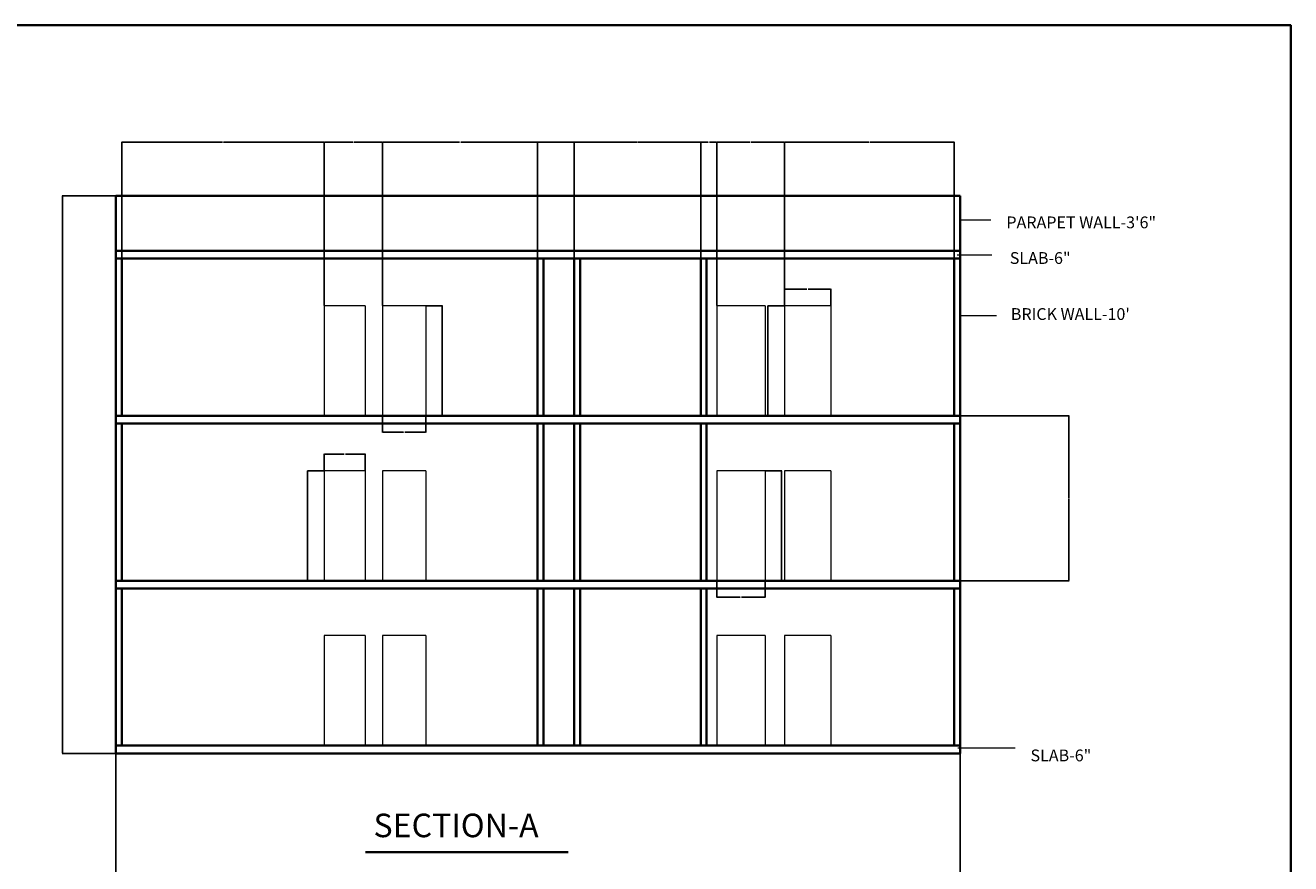
# Model space of a CAD drawing. Units: inches. Extents: x 1520 to 3401, y 1570 to 3432.
# Tile 15 of 15: x 2435 to 3401, y 2791 to 3432. Entities that reach past the tile are written whole.
import ezdxf

# ---------------------------------------------------------------- set-up
doc = ezdxf.new("R2010")
doc.units = ezdxf.units.IN
for name, color, linetype, lineweight in [('A-ANNO-DIMS', 2, 'Continuous', 18), ('A-ANNO-TEXT', 7, 'Continuous', 18), ('A-ANNO-TITL', 7, 'Continuous', 35), ('A-ANNO-TTLB', 7, 'Continuous', 35), ('A-SECT', 7, 'Continuous', 35), ('A-SECT-DOOR', 3, 'Continuous', 18), ('A-SECT-SLAB', 7, 'Continuous', 35)]:
    doc.layers.add(name, color=color, linetype=linetype, lineweight=lineweight)
doc.styles.get("Standard").update_dxf_attribs({"font": 'arial.ttf'})
doc.dimstyles.get("Standard").update_dxf_attribs({"dimtxt": 0.18, "dimasz": 0.18, "dimexe": 0.18, "dimexo": 0.0625, "dimgap": 0.09, "dimtad": 0, "dimtih": 1, "dimtoh": 1, "dimdec": 4, "dimzin": 0, "dimdsep": 46, "dimtxsty": 'Standard', "dimcen": 0.09, "dimadec": 0, "dimazin": 0, "dimtfac": 1, "dimtdec": 4, "dimtofl": 0, "dimtmove": 0, "dimatfit": 3, "dimfxl": 1, "dimtolj": 1, "dimtzin": 0, "dimarcsym": 0})

# ---------------------------------------------------------------- blocks, each defined once
blk = doc.blocks.new('DOOR-SECT-01')
for p, q in [((0, 84), (0, 0)), ((31.45, 84), (0, 84)), ((31.45, 84), (31.45, 0))]:
    blk.add_line(p, q)
blk = doc.blocks.new('DOOR-SECT-02')
for p, q in [((0, 84), (0, 0)), ((32.99, 84), (0, 84)), ((32.99, 84), (32.99, 0))]:
    blk.add_line(p, q)
blk = doc.blocks.new('DOOR-SECT-03')
for p, q in [((0, 84), (0, 0)), ((36.83, 84), (0, 84)), ((36.83, 84), (36.83, 0))]:
    blk.add_line(p, q)
blk = doc.blocks.new('DOOR-SECT-04')
for p, q in [((0, 84), (0, 0)), ((35.31, 84), (0, 84)), ((35.31, 84), (35.31, 0))]:
    blk.add_line(p, q)
blk = doc.blocks.new('*D73')
at = {"layer": 'A-ANNO-DIMS', "color": 0, "lineweight": -2, "transparency": 16777216}
for p, q in [((2662.81, 3091.63), (2650.09, 3091.63)), ((2650.27, 3091.45), (2650.27, 3049.82)), ((2650.27, 3007.81), (2650.27, 3049.45)), ((2662.81, 3007.63), (2650.09, 3007.63))]:
    blk.add_line(p, q, dxfattribs=at)
at = {"layer": 'A-ANNO-DIMS', "color": 0, "transparency": 16777216}
for points in [[(2650.24, 3091.45), (2650.3, 3091.45), (2650.27, 3091.63)], [(2650.24, 3007.81), (2650.3, 3007.81), (2650.27, 3007.63)]]:
    blk.add_solid(points, dxfattribs=at)
at = {"layer": 'Defpoints', "color": 0, "transparency": 16777216}
for p in [(2650.27, 3091.63), (2662.87, 3091.63), (2662.87, 3007.63)]:
    blk.add_point(p, dxfattribs=at)
at = {"layer": 'A-ANNO-DIMS', "color": 0, "transparency": 16777216, "insert": (2650.27, 3049.63), "char_height": 0.18, "attachment_point": 5}
blk.add_mtext('\\A1;S1 84 TYP.', dxfattribs=at)
blk = doc.blocks.new('*D74')
at = {"layer": 'A-ANNO-DIMS', "color": 0, "lineweight": -2, "transparency": 16777216}
for p, q in [((2662.87, 3091.7), (2662.87, 3104.41)), ((2663.05, 3104.23), (2678.07, 3104.23)), ((2694.14, 3104.23), (2679.12, 3104.23)), ((2694.32, 3091.7), (2694.32, 3104.41))]:
    blk.add_line(p, q, dxfattribs=at)
at = {"layer": 'A-ANNO-DIMS', "color": 0, "transparency": 16777216}
for points in [[(2663.05, 3104.26), (2663.05, 3104.2), (2662.87, 3104.23)], [(2694.14, 3104.26), (2694.14, 3104.2), (2694.32, 3104.23)]]:
    blk.add_solid(points, dxfattribs=at)
at = {"layer": 'Defpoints', "color": 0, "transparency": 16777216}
for p in [(2694.32, 3104.23), (2662.87, 3091.63), (2694.32, 3091.63)]:
    blk.add_point(p, dxfattribs=at)
at = {"layer": 'A-ANNO-DIMS', "color": 0, "transparency": 16777216, "insert": (2678.6, 3104.23), "char_height": 0.18, "attachment_point": 5}
blk.add_mtext('\\A1;31 TYP.', dxfattribs=at)
blk = doc.blocks.new('*D75')
at = {"layer": 'A-ANNO-DIMS', "color": 0, "lineweight": -2, "transparency": 16777216}
for p, q in [((2740.5, 3217.63), (2753.22, 3217.63)), ((2753.04, 3217.45), (2753.04, 3175.82)), ((2753.04, 3133.81), (2753.04, 3175.45)), ((2740.5, 3133.63), (2753.22, 3133.63))]:
    blk.add_line(p, q, dxfattribs=at)
at = {"layer": 'A-ANNO-DIMS', "color": 0, "transparency": 16777216}
for points in [[(2753.01, 3217.45), (2753.07, 3217.45), (2753.04, 3217.63)], [(2753.01, 3133.81), (2753.07, 3133.81), (2753.04, 3133.63)]]:
    blk.add_solid(points, dxfattribs=at)
at = {"layer": 'Defpoints', "color": 0, "transparency": 16777216}
for p in [(2740.44, 3217.63), (2753.04, 3217.63), (2740.44, 3133.63)]:
    blk.add_point(p, dxfattribs=at)
at = {"layer": 'A-ANNO-DIMS', "color": 0, "transparency": 16777216, "insert": (2753.04, 3175.63), "char_height": 0.18, "attachment_point": 5}
blk.add_mtext('\\A1;S2 84 TYP.', dxfattribs=at)
blk = doc.blocks.new('*D76')
at = {"layer": 'A-ANNO-DIMS', "color": 0, "lineweight": -2, "transparency": 16777216}
for p, q in [((2707.45, 3133.57), (2707.45, 3120.85)), ((2740.44, 3133.57), (2740.44, 3120.85)), ((2707.63, 3121.03), (2723.42, 3121.03)), ((2740.26, 3121.03), (2724.47, 3121.03))]:
    blk.add_line(p, q, dxfattribs=at)
at = {"layer": 'A-ANNO-DIMS', "color": 0, "transparency": 16777216}
for points in [[(2707.63, 3121.06), (2707.63, 3121), (2707.45, 3121.03)], [(2740.26, 3121.06), (2740.26, 3121), (2740.44, 3121.03)]]:
    blk.add_solid(points, dxfattribs=at)
at = {"layer": 'Defpoints', "color": 0, "transparency": 16777216}
for p in [(2707.45, 3133.63), (2740.44, 3133.63), (2740.44, 3121.03)]:
    blk.add_point(p, dxfattribs=at)
at = {"layer": 'A-ANNO-DIMS', "color": 0, "transparency": 16777216, "insert": (2723.95, 3121.03), "char_height": 0.18, "attachment_point": 5}
blk.add_mtext('\\A1;33 TYP.', dxfattribs=at)
blk = doc.blocks.new('*D77')
at = {"layer": 'A-ANNO-DIMS', "color": 0, "lineweight": -2, "transparency": 16777216}
for p, q in [((2999.61, 3091.63), (3012.33, 3091.63)), ((3012.15, 3091.45), (3012.15, 3049.82)), ((3012.15, 3007.81), (3012.15, 3049.45)), ((2999.61, 3007.63), (3012.33, 3007.63))]:
    blk.add_line(p, q, dxfattribs=at)
at = {"layer": 'A-ANNO-DIMS', "color": 0, "transparency": 16777216}
for points in [[(3012.12, 3091.45), (3012.18, 3091.45), (3012.15, 3091.63)], [(3012.12, 3007.81), (3012.18, 3007.81), (3012.15, 3007.63)]]:
    blk.add_solid(points, dxfattribs=at)
at = {"layer": 'Defpoints', "color": 0, "transparency": 16777216}
for p in [(2999.55, 3091.63), (3012.15, 3091.63), (2999.55, 3007.63)]:
    blk.add_point(p, dxfattribs=at)
at = {"layer": 'A-ANNO-DIMS', "color": 0, "transparency": 16777216, "insert": (3012.15, 3049.63), "char_height": 0.18, "attachment_point": 5}
blk.add_mtext('\\A1;S3 84 TYP.', dxfattribs=at)
blk = doc.blocks.new('*D78')
at = {"layer": 'A-ANNO-DIMS', "color": 0, "lineweight": -2, "transparency": 16777216}
for p, q in [((2962.72, 3007.57), (2962.72, 2994.85)), ((2999.55, 3007.57), (2999.55, 2994.85)), ((2962.9, 2995.03), (2980.61, 2995.03)), ((2999.37, 2995.03), (2981.66, 2995.03))]:
    blk.add_line(p, q, dxfattribs=at)
at = {"layer": 'A-ANNO-DIMS', "color": 0, "transparency": 16777216}
for points in [[(2962.9, 2995.06), (2962.9, 2995), (2962.72, 2995.03)], [(2999.37, 2995.06), (2999.37, 2995), (2999.55, 2995.03)]]:
    blk.add_solid(points, dxfattribs=at)
at = {"layer": 'Defpoints', "color": 0, "transparency": 16777216}
for p in [(2962.72, 3007.63), (2999.55, 3007.63), (2999.55, 2995.03)]:
    blk.add_point(p, dxfattribs=at)
at = {"layer": 'A-ANNO-DIMS', "color": 0, "transparency": 16777216, "insert": (2981.14, 2995.03), "char_height": 0.18, "attachment_point": 5}
blk.add_mtext('\\A1;37 TYP.', dxfattribs=at)
blk = doc.blocks.new('*D79')
at = {"layer": 'A-ANNO-DIMS', "color": 0, "lineweight": -2, "transparency": 16777216}
for p, q in [((3014.28, 3217.63), (3001.56, 3217.63)), ((3001.74, 3217.45), (3001.74, 3175.82)), ((3001.74, 3133.81), (3001.74, 3175.45)), ((3014.28, 3133.63), (3001.56, 3133.63))]:
    blk.add_line(p, q, dxfattribs=at)
at = {"layer": 'A-ANNO-DIMS', "color": 0, "transparency": 16777216}
for points in [[(3001.71, 3217.45), (3001.77, 3217.45), (3001.74, 3217.63)], [(3001.71, 3133.81), (3001.77, 3133.81), (3001.74, 3133.63)]]:
    blk.add_solid(points, dxfattribs=at)
at = {"layer": 'Defpoints', "color": 0, "transparency": 16777216}
for p in [(3001.74, 3217.63), (3014.34, 3217.63), (3014.34, 3133.63)]:
    blk.add_point(p, dxfattribs=at)
at = {"layer": 'A-ANNO-DIMS', "color": 0, "transparency": 16777216, "insert": (3001.74, 3175.63), "char_height": 0.18, "attachment_point": 5}
blk.add_mtext('\\A1;S4 84 TYP.', dxfattribs=at)
blk = doc.blocks.new('*D80')
at = {"layer": 'A-ANNO-DIMS', "color": 0, "lineweight": -2, "transparency": 16777216}
for p, q in [((3014.34, 3217.7), (3014.34, 3230.41)), ((3014.52, 3230.23), (3031.47, 3230.23)), ((3049.47, 3230.23), (3032.52, 3230.23)), ((3049.65, 3217.7), (3049.65, 3230.41))]:
    blk.add_line(p, q, dxfattribs=at)
at = {"layer": 'A-ANNO-DIMS', "color": 0, "transparency": 16777216}
for points in [[(3014.52, 3230.26), (3014.52, 3230.2), (3014.34, 3230.23)], [(3049.47, 3230.26), (3049.47, 3230.2), (3049.65, 3230.23)]]:
    blk.add_solid(points, dxfattribs=at)
at = {"layer": 'Defpoints', "color": 0, "transparency": 16777216}
for p in [(3049.65, 3230.23), (3014.34, 3217.63), (3049.65, 3217.63)]:
    blk.add_point(p, dxfattribs=at)
at = {"layer": 'A-ANNO-DIMS', "color": 0, "transparency": 16777216, "insert": (3032, 3230.23), "char_height": 0.18, "attachment_point": 5}
blk.add_mtext('\\A1;35 TYP.', dxfattribs=at)
blk = doc.blocks.new('*D211')
at = {"layer": 'A-ANNO-DIMS', "color": 0, "lineweight": -2, "transparency": 16777216}
for p, q in [((3148.46, 3133.63), (3231.65, 3133.63)), ((3231.47, 3133.45), (3231.47, 3070.81)), ((3231.47, 3007.81), (3231.47, 3070.45)), ((3148.46, 3007.63), (3231.65, 3007.63))]:
    blk.add_line(p, q, dxfattribs=at)
at = {"layer": 'A-ANNO-DIMS', "color": 0, "transparency": 16777216}
for points in [[(3231.44, 3133.45), (3231.5, 3133.45), (3231.47, 3133.63)], [(3231.44, 3007.81), (3231.5, 3007.81), (3231.47, 3007.63)]]:
    blk.add_solid(points, dxfattribs=at)
at = {"layer": 'Defpoints', "color": 0, "transparency": 16777216}
for p in [(3148.4, 3133.63), (3231.47, 3133.63), (3148.4, 3007.63)]:
    blk.add_point(p, dxfattribs=at)
at = {"layer": 'A-ANNO-DIMS', "color": 0, "transparency": 16777216, "insert": (3231.47, 3070.63), "char_height": 0.18, "attachment_point": 5}
blk.add_mtext('\\A1;126', dxfattribs=at)
blk = doc.blocks.new('*D224')
at = {"layer": 'A-ANNO-DIMS', "color": 0, "lineweight": -2, "transparency": 16777216}
for p, q in [((2503.9, 2875.57), (2503.9, 2759.2)), ((3148.4, 2875.57), (3148.4, 2759.2)), ((2504.08, 2759.38), (2825.75, 2759.38)), ((3148.22, 2759.38), (2826.54, 2759.38))]:
    blk.add_line(p, q, dxfattribs=at)
at = {"layer": 'A-ANNO-DIMS', "color": 0, "transparency": 16777216}
for points in [[(2504.08, 2759.41), (2504.08, 2759.35), (2503.9, 2759.38)], [(3148.22, 2759.41), (3148.22, 2759.35), (3148.4, 2759.38)]]:
    blk.add_solid(points, dxfattribs=at)
at = {"layer": 'Defpoints', "color": 0, "transparency": 16777216}
for p in [(2503.9, 2875.63), (3148.4, 2875.63), (3148.4, 2759.38)]:
    blk.add_point(p, dxfattribs=at)
at = {"layer": 'A-ANNO-DIMS', "color": 0, "transparency": 16777216, "insert": (2826.15, 2759.38), "char_height": 0.18, "attachment_point": 5}
blk.add_mtext('\\A1;644.5', dxfattribs=at)
blk = doc.blocks.new('*D225')
at = {"layer": 'A-ANNO-DIMS', "color": 0, "lineweight": -2, "transparency": 16777216}
for p, q in [((2503.84, 3301.63), (2462.87, 3301.63)), ((2463.05, 3301.45), (2463.05, 3088.81)), ((2463.05, 2875.81), (2463.05, 3088.45)), ((2503.84, 2875.63), (2462.87, 2875.63))]:
    blk.add_line(p, q, dxfattribs=at)
at = {"layer": 'A-ANNO-DIMS', "color": 0, "transparency": 16777216}
for points in [[(2463.02, 3301.45), (2463.08, 3301.45), (2463.05, 3301.63)], [(2463.02, 2875.81), (2463.08, 2875.81), (2463.05, 2875.63)]]:
    blk.add_solid(points, dxfattribs=at)
at = {"layer": 'Defpoints', "color": 0, "transparency": 16777216}
for p in [(2503.9, 3301.63), (2463.05, 2875.63), (2503.9, 2875.63)]:
    blk.add_point(p, dxfattribs=at)
at = {"layer": 'A-ANNO-DIMS', "color": 0, "transparency": 16777216, "insert": (2463.05, 3088.63), "char_height": 0.18, "attachment_point": 5}
blk.add_mtext('\\A1;426', dxfattribs=at)
blk = doc.blocks.new('*D226')
at = {"layer": 'A-ANNO-DIMS', "color": 0, "lineweight": -2, "transparency": 16777216}
for p, q in [((2508.4, 3253.7), (2508.4, 3342.66)), ((2508.58, 3342.48), (2585.18, 3342.48)), ((2662.69, 3342.48), (2586.09, 3342.48)), ((2662.87, 3217.7), (2662.87, 3342.66))]:
    blk.add_line(p, q, dxfattribs=at)
at = {"layer": 'A-ANNO-DIMS', "color": 0, "transparency": 16777216}
for points in [[(2508.58, 3342.51), (2508.58, 3342.45), (2508.4, 3342.48)], [(2662.69, 3342.51), (2662.69, 3342.45), (2662.87, 3342.48)]]:
    blk.add_solid(points, dxfattribs=at)
at = {"layer": 'Defpoints', "color": 0, "transparency": 16777216}
for p in [(2662.87, 3342.48), (2508.4, 3253.63), (2662.87, 3217.63)]:
    blk.add_point(p, dxfattribs=at)
at = {"layer": 'A-ANNO-DIMS', "color": 0, "transparency": 16777216, "insert": (2585.64, 3342.48), "char_height": 0.18, "attachment_point": 5}
blk.add_mtext('\\A1;154.47', dxfattribs=at)
blk = doc.blocks.new('*D227')
at = {"layer": 'A-ANNO-DIMS', "color": 0, "lineweight": -2, "transparency": 16777216}
for p, q in [((2662.87, 3217.7), (2662.87, 3342.66)), ((2663.05, 3342.48), (2684.76, 3342.48)), ((2707.27, 3342.48), (2685.56, 3342.48)), ((2707.45, 3217.7), (2707.45, 3342.66))]:
    blk.add_line(p, q, dxfattribs=at)
at = {"layer": 'A-ANNO-DIMS', "color": 0, "transparency": 16777216}
for points in [[(2663.05, 3342.51), (2663.05, 3342.45), (2662.87, 3342.48)], [(2707.27, 3342.51), (2707.27, 3342.45), (2707.45, 3342.48)]]:
    blk.add_solid(points, dxfattribs=at)
at = {"layer": 'Defpoints', "color": 0, "transparency": 16777216}
for p in [(2707.45, 3342.48), (2662.87, 3217.63), (2707.45, 3217.63)]:
    blk.add_point(p, dxfattribs=at)
at = {"layer": 'A-ANNO-DIMS', "color": 0, "transparency": 16777216, "insert": (2685.16, 3342.48), "char_height": 0.18, "attachment_point": 5}
blk.add_mtext('\\A1;44.58', dxfattribs=at)
blk = doc.blocks.new('*D228')
at = {"layer": 'A-ANNO-DIMS', "color": 0, "lineweight": -2, "transparency": 16777216}
for p, q in [((2707.45, 3217.7), (2707.45, 3342.66)), ((2707.63, 3342.48), (2766.22, 3342.48)), ((2825.72, 3342.48), (2767.13, 3342.48)), ((2825.9, 3253.7), (2825.9, 3342.66))]:
    blk.add_line(p, q, dxfattribs=at)
at = {"layer": 'A-ANNO-DIMS', "color": 0, "transparency": 16777216}
for points in [[(2707.63, 3342.51), (2707.63, 3342.45), (2707.45, 3342.48)], [(2825.72, 3342.51), (2825.72, 3342.45), (2825.9, 3342.48)]]:
    blk.add_solid(points, dxfattribs=at)
at = {"layer": 'Defpoints', "color": 0, "transparency": 16777216}
for p in [(2825.9, 3342.48), (2825.9, 3253.63), (2707.45, 3217.63)]:
    blk.add_point(p, dxfattribs=at)
at = {"layer": 'A-ANNO-DIMS', "color": 0, "transparency": 16777216, "insert": (2766.67, 3342.48), "char_height": 0.18, "attachment_point": 5}
blk.add_mtext('\\A1;118.45', dxfattribs=at)
blk = doc.blocks.new('*D229')
at = {"layer": 'A-ANNO-DIMS', "color": 0, "lineweight": -2, "transparency": 16777216}
for p, q in [((2825.9, 3253.7), (2825.9, 3342.66)), ((2826.08, 3342.48), (2839.68, 3342.48)), ((2853.72, 3342.48), (2840.12, 3342.48)), ((2853.9, 3253.7), (2853.9, 3342.66))]:
    blk.add_line(p, q, dxfattribs=at)
at = {"layer": 'A-ANNO-DIMS', "color": 0, "transparency": 16777216}
for points in [[(2826.08, 3342.51), (2826.08, 3342.45), (2825.9, 3342.48)], [(2853.72, 3342.51), (2853.72, 3342.45), (2853.9, 3342.48)]]:
    blk.add_solid(points, dxfattribs=at)
at = {"layer": 'Defpoints', "color": 0, "transparency": 16777216}
for p in [(2853.9, 3342.48), (2825.9, 3253.63), (2853.9, 3253.63)]:
    blk.add_point(p, dxfattribs=at)
at = {"layer": 'A-ANNO-DIMS', "color": 0, "transparency": 16777216, "insert": (2839.9, 3342.48), "char_height": 0.18, "attachment_point": 5}
blk.add_mtext('\\A1;28', dxfattribs=at)
blk = doc.blocks.new('*D230')
at = {"layer": 'A-ANNO-DIMS', "color": 0, "lineweight": -2, "transparency": 16777216}
for p, q in [((2853.9, 3253.7), (2853.9, 3342.66)), ((2854.08, 3342.48), (2901.82, 3342.48)), ((2950.22, 3342.48), (2902.47, 3342.48)), ((2950.4, 3253.7), (2950.4, 3342.66))]:
    blk.add_line(p, q, dxfattribs=at)
at = {"layer": 'A-ANNO-DIMS', "color": 0, "transparency": 16777216}
for points in [[(2854.08, 3342.51), (2854.08, 3342.45), (2853.9, 3342.48)], [(2950.22, 3342.51), (2950.22, 3342.45), (2950.4, 3342.48)]]:
    blk.add_solid(points, dxfattribs=at)
at = {"layer": 'Defpoints', "color": 0, "transparency": 16777216}
for p in [(2950.4, 3342.48), (2853.9, 3253.63), (2950.4, 3253.63)]:
    blk.add_point(p, dxfattribs=at)
at = {"layer": 'A-ANNO-DIMS', "color": 0, "transparency": 16777216, "insert": (2902.15, 3342.48), "char_height": 0.18, "attachment_point": 5}
blk.add_mtext('\\A1;96.5', dxfattribs=at)
blk = doc.blocks.new('*D231')
at = {"layer": 'A-ANNO-DIMS', "color": 0, "lineweight": -2, "transparency": 16777216}
for p, q in [((2950.4, 3253.7), (2950.4, 3342.66)), ((2950.58, 3342.48), (2956.11, 3342.48)), ((2962.54, 3342.48), (2957.01, 3342.48)), ((2962.72, 3217.7), (2962.72, 3342.66))]:
    blk.add_line(p, q, dxfattribs=at)
at = {"layer": 'A-ANNO-DIMS', "color": 0, "transparency": 16777216}
for points in [[(2950.58, 3342.51), (2950.58, 3342.45), (2950.4, 3342.48)], [(2962.54, 3342.51), (2962.54, 3342.45), (2962.72, 3342.48)]]:
    blk.add_solid(points, dxfattribs=at)
at = {"layer": 'Defpoints', "color": 0, "transparency": 16777216}
for p in [(2962.72, 3342.48), (2950.4, 3253.63), (2962.72, 3217.63)]:
    blk.add_point(p, dxfattribs=at)
at = {"layer": 'A-ANNO-DIMS', "color": 0, "transparency": 16777216, "insert": (2956.56, 3342.48), "char_height": 0.18, "attachment_point": 5}
blk.add_mtext('\\A1;12.322', dxfattribs=at)
blk = doc.blocks.new('*D232')
at = {"layer": 'A-ANNO-DIMS', "color": 0, "lineweight": -2, "transparency": 16777216}
for p, q in [((2962.72, 3217.7), (2962.72, 3342.66)), ((2962.9, 3342.48), (2988.14, 3342.48)), ((3014.16, 3342.48), (2988.92, 3342.48)), ((3014.34, 3217.7), (3014.34, 3342.66))]:
    blk.add_line(p, q, dxfattribs=at)
at = {"layer": 'A-ANNO-DIMS', "color": 0, "transparency": 16777216}
for points in [[(2962.9, 3342.51), (2962.9, 3342.45), (2962.72, 3342.48)], [(3014.16, 3342.51), (3014.16, 3342.45), (3014.34, 3342.48)]]:
    blk.add_solid(points, dxfattribs=at)
at = {"layer": 'Defpoints', "color": 0, "transparency": 16777216}
for p in [(3014.34, 3342.48), (2962.72, 3217.63), (3014.34, 3217.63)]:
    blk.add_point(p, dxfattribs=at)
at = {"layer": 'A-ANNO-DIMS', "color": 0, "transparency": 16777216, "insert": (2988.53, 3342.48), "char_height": 0.18, "attachment_point": 5}
blk.add_mtext('\\A1;51.62', dxfattribs=at)
blk = doc.blocks.new('*D233')
at = {"layer": 'A-ANNO-DIMS', "color": 0, "lineweight": -2, "transparency": 16777216}
for p, q in [((3014.34, 3217.7), (3014.34, 3342.66)), ((3014.52, 3342.48), (3078.66, 3342.48)), ((3143.72, 3342.48), (3079.57, 3342.48)), ((3143.9, 3253.7), (3143.9, 3342.66))]:
    blk.add_line(p, q, dxfattribs=at)
at = {"layer": 'A-ANNO-DIMS', "color": 0, "transparency": 16777216}
for points in [[(3014.52, 3342.51), (3014.52, 3342.45), (3014.34, 3342.48)], [(3143.72, 3342.51), (3143.72, 3342.45), (3143.9, 3342.48)]]:
    blk.add_solid(points, dxfattribs=at)
at = {"layer": 'Defpoints', "color": 0, "transparency": 16777216}
for p in [(3143.9, 3342.48), (3143.9, 3253.63), (3014.34, 3217.63)]:
    blk.add_point(p, dxfattribs=at)
at = {"layer": 'A-ANNO-DIMS', "color": 0, "transparency": 16777216, "insert": (3079.12, 3342.48), "char_height": 0.18, "attachment_point": 5}
blk.add_mtext('\\A1;129.56', dxfattribs=at)

msp = doc.modelspace()

# ---------------------------------------------------------------- linework, layer by layer
at = {"layer": 'A-ANNO-TEXT'}
for p, q in [((3148.3987, 3283.1525), (3172.0389, 3283.1525)), ((3146.3387, 3256.5408), (3172.5644, 3256.5408)), ((3148.3987, 3210.133), (3176.2149, 3210.133)), ((3146.6484, 2880.0126), (3190.6167, 2880.0126))]:
    msp.add_line(p, q, dxfattribs=at)
at = {"layer": 'A-ANNO-TITL'}
msp.add_line((2694.4227, 2800.2305), (2849.109, 2800.2305), dxfattribs=at)
at = {"layer": 'A-ANNO-TTLB'}
msp.add_lwpolyline([(1519.9253, 3431.7421), (3400.8761, 3431.7421), (3400.8761, 1570.3458), (1519.9253, 1570.3458)], close=True, dxfattribs=at)
at = {"layer": 'A-SECT'}
for p, q in [((2503.8987, 3301.633), (2503.8987, 3118.633)), ((3148.3987, 3301.633), (2503.8987, 3301.633)), ((3148.3987, 3301.633), (3148.3987, 3118.633)), ((2508.3987, 3253.633), (2508.3987, 3133.633)), ((2825.8987, 3253.633), (2825.8987, 3133.633)), ((2830.3987, 3253.633), (2830.3987, 3133.633)), ((2853.8987, 3253.633), (2853.8987, 3133.633)), ((2858.3987, 3253.633), (2858.3987, 3133.633)), ((2950.3987, 3253.633), (2950.3987, 3133.633)), ((2954.8987, 3253.633), (2954.8987, 3133.633)), ((3143.8987, 3253.633), (3143.8987, 3133.633)), ((2503.8987, 3175.633), (2503.8987, 2992.633)), ((3148.3987, 3175.633), (3148.3987, 2992.633)), ((2508.3987, 3127.633), (2508.3987, 3007.633)), ((2825.8987, 3127.633), (2825.8987, 3007.633)), ((2830.3987, 3127.633), (2830.3987, 3007.633)), ((2853.8987, 3127.633), (2853.8987, 3007.633)), ((2858.3987, 3127.633), (2858.3987, 3007.633)), ((2950.3987, 3127.633), (2950.3987, 3007.633)), ((2954.8987, 3127.633), (2954.8987, 3007.633)), ((3143.8987, 3127.633), (3143.8987, 3007.633)), ((2503.8987, 3049.633), (2503.8987, 2875.633)), ((3148.3987, 3049.633), (3148.3987, 2875.633)), ((2508.3987, 3001.633), (2508.3987, 2881.633)), ((2825.8987, 3001.633), (2825.8987, 2881.633)), ((2830.3987, 3001.633), (2830.3987, 2881.633)), ((2853.8987, 3001.633), (2853.8987, 2881.633)), ((2858.3987, 3001.633), (2858.3987, 2881.633)), ((2950.3987, 3001.633), (2950.3987, 2881.633)), ((2954.8987, 3001.633), (2954.8987, 2881.633)), ((3143.8987, 3001.633), (3143.8987, 2881.633))]:
    msp.add_line(p, q, dxfattribs=at)
at = {"layer": 'A-SECT-SLAB'}
for p, q in [((3148.3987, 3259.633), (2503.8987, 3259.633)), ((3148.3987, 3253.633), (2503.8987, 3253.633)), ((3148.3987, 3133.633), (2503.8987, 3133.633)), ((3148.3987, 3127.633), (2503.8987, 3127.633)), ((3148.3987, 3007.633), (2503.8987, 3007.633)), ((3148.3987, 3001.633), (2503.8987, 3001.633)), ((3148.3987, 2881.633), (2503.8987, 2881.633)), ((2503.8987, 2881.633), (2503.8987, 2875.633)), ((2503.8987, 2875.633), (3148.3987, 2875.633))]:
    msp.add_line(p, q, dxfattribs=at)

# ---------------------------------------------------------------- block references
at = {"layer": 'A-SECT-DOOR'}
for name, p in [('DOOR-SECT-01', (2662.872, 3133.633)), ('DOOR-SECT-02', (2707.45, 3133.633)), ('DOOR-SECT-03', (2962.721, 3133.633)), ('DOOR-SECT-04', (3014.339, 3133.633)), ('DOOR-SECT-01', (2662.872, 3007.633)), ('DOOR-SECT-02', (2707.45, 3007.633)), ('DOOR-SECT-03', (2962.721, 3007.633)), ('DOOR-SECT-04', (3014.339, 3007.633)), ('DOOR-SECT-01', (2662.872, 2881.633)), ('DOOR-SECT-02', (2707.45, 2881.633)), ('DOOR-SECT-03', (2962.721, 2881.633)), ('DOOR-SECT-04', (3014.339, 2881.633))]:
    msp.add_blockref(name, p, dxfattribs=at)

# ---------------------------------------------------------------- texts
at = {"layer": 'A-ANNO-TEXT', "char_height": 9, "attachment_point": 1}
for s, width, insert in [('PARAPET WALL-3\'6"', 157.514715, (3183.7912, 3285.737)), ('SLAB-6"', 69.827308, (3186.408, 3258.5154)), ("BRICK WALL-10'", 119.022415, (3187.2042, 3215.7334)), ('SLAB-6"', 172.572429, (3202.2165, 2878.6762))]:
    msp.add_mtext_dynamic_manual_height_columns(s, width=width, gutter_width=12.5, heights=[0], dxfattribs=dict(at, insert=insert))
at = {"layer": 'A-ANNO-TITL', "insert": (2700.5449, 2829.7208), "char_height": 18, "attachment_point": 1}
msp.add_mtext_dynamic_manual_height_columns('SECTION-A', width=303.339366, gutter_width=12.5, heights=[0], dxfattribs=at)

# ---------------------------------------------------------------- dimensions: what is measured, and where the dimension line sits
at = {"layer": 'A-ANNO-DIMS'}
for base, p1, p2, override, picture, middle in [((2662.8719, 3342.483), (2508.3987, 3253.633), (2662.8719, 3217.633), {"dimdec": 2, "dimlfac": 1, "dimrnd": 0, "dimzin": 0, "dimdsep": 46, "dimlunit": 2}, '*D226', (2585.6353, 3342.483)), ((2707.4502, 3342.483), (2662.8719, 3217.633), (2707.4502, 3217.633), {"dimdec": 2, "dimlfac": 1, "dimrnd": 0, "dimzin": 0, "dimdsep": 46, "dimlunit": 2}, '*D227', (2685.161, 3342.483)), ((2825.8987, 3342.483), (2707.4502, 3217.633), (2825.8987, 3253.633), {"dimdec": 2, "dimlfac": 1, "dimrnd": 0, "dimzin": 0, "dimdsep": 46, "dimlunit": 2}, '*D228', (2766.6744, 3342.483)), ((2853.8987, 3342.483), (2825.8987, 3253.633), (2853.8987, 3253.633), {"dimdec": 0, "dimlfac": 1, "dimrnd": 0, "dimzin": 0, "dimdsep": 46, "dimlunit": 2}, '*D229', (2839.8987, 3342.483)), ((2950.3987, 3342.483), (2853.8987, 3253.633), (2950.3987, 3253.633), {"dimdec": 1, "dimlfac": 1, "dimrnd": 0, "dimzin": 0, "dimdsep": 46, "dimlunit": 2}, '*D230', (2902.1487, 3342.483)), ((2962.7207, 3342.483), (2950.3987, 3253.633), (2962.7207, 3217.633), {"dimdec": 3, "dimlfac": 1, "dimrnd": 0, "dimzin": 0, "dimdsep": 46, "dimlunit": 2}, '*D231', (2956.5597, 3342.483)), ((3014.3386, 3342.483), (2962.7207, 3217.633), (3014.3386, 3217.633), {"dimdec": 2, "dimlfac": 1, "dimrnd": 0, "dimzin": 0, "dimdsep": 46, "dimlunit": 2}, '*D232', (2988.5296, 3342.483)), ((3143.8987, 3342.483), (3014.3386, 3217.633), (3143.8987, 3253.633), {"dimdec": 2, "dimlfac": 1, "dimrnd": 0, "dimzin": 0, "dimdsep": 46, "dimlunit": 2}, '*D233', (3079.1186, 3342.483)), ((3148.3987, 2759.3805), (2503.8987, 2875.633), (3148.3987, 2875.633), {"dimdec": 1, "dimlfac": 1, "dimrnd": 0, "dimzin": 0, "dimdsep": 46, "dimlunit": 2}, '*D224', (2826.1487, 2759.3805))]:
    dim = msp.add_linear_dim(base=base, p1=p1, p2=p2, dimstyle='Standard', override=override, dxfattribs=at)
    dim.commit()
    dim.dimension.update_dxf_attribs({"geometry": picture, "text_midpoint": middle})
for base, p1, p2, picture, middle in [((2463.0487, 2875.633), (2503.8987, 3301.633), (2503.8987, 2875.633), '*D225', (2463.0487, 3088.633)), ((3231.4667, 3133.633), (3148.3987, 3007.633), (3148.3987, 3133.633), '*D211', (3231.4667, 3070.633))]:
    dim = msp.add_linear_dim(base=base, p1=p1, p2=p2, angle=90, dimstyle='Standard', override={"dimdec": 0, "dimlfac": 1, "dimrnd": 0, "dimzin": 0, "dimdsep": 46, "dimlunit": 2}, dxfattribs=at)
    dim.commit()
    dim.dimension.update_dxf_attribs({"geometry": picture, "text_midpoint": middle})
for base, p1, p2, picture, middle in [((3049.6534, 3230.233), (3014.3386, 3217.633), (3049.6534, 3217.633), '*D80', (3031.996, 3230.233)), ((2740.4425, 3121.033), (2707.4502, 3133.633), (2740.4425, 3133.633), '*D76', (2723.9463, 3121.033)), ((2694.3184, 3104.233), (2662.8719, 3091.633), (2694.3184, 3091.633), '*D74', (2678.5951, 3104.233)), ((2999.5513, 2995.033), (2962.7207, 3007.633), (2999.5513, 3007.633), '*D78', (2981.136, 2995.033))]:
    dim = msp.add_linear_dim(base=base, p1=p1, p2=p2, text='<> TYP.', dimstyle='Standard', override={"dimdec": 0, "dimlfac": 1, "dimrnd": 0, "dimzin": 0, "dimdsep": 46, "dimlunit": 2}, dxfattribs=at)
    dim.commit()
    dim.dimension.update_dxf_attribs({"geometry": picture, "text_midpoint": middle})
for base, p1, p2, text, picture, middle in [((2753.0425, 3217.633), (2740.4425, 3133.633), (2740.4425, 3217.633), 'S2 <> TYP.', '*D75', (2753.0425, 3175.633)), ((3001.7386, 3217.633), (3014.3386, 3133.633), (3014.3386, 3217.633), 'S4 <> TYP.', '*D79', (3001.7386, 3175.633)), ((2650.2719, 3091.633), (2662.8719, 3007.633), (2662.8719, 3091.633), 'S1 <> TYP.', '*D73', (2650.2719, 3049.633)), ((3012.1513, 3091.633), (2999.5513, 3007.633), (2999.5513, 3091.633), 'S3 <> TYP.', '*D77', (3012.1513, 3049.633))]:
    dim = msp.add_linear_dim(base=base, p1=p1, p2=p2, angle=90, text=text, dimstyle='Standard', override={"dimdec": 0, "dimlfac": 1, "dimrnd": 0, "dimzin": 0, "dimdsep": 46, "dimlunit": 2}, dxfattribs=at)
    dim.commit()
    dim.dimension.update_dxf_attribs({"geometry": picture, "text_midpoint": middle})

doc.saveas('drawing.dxf')
